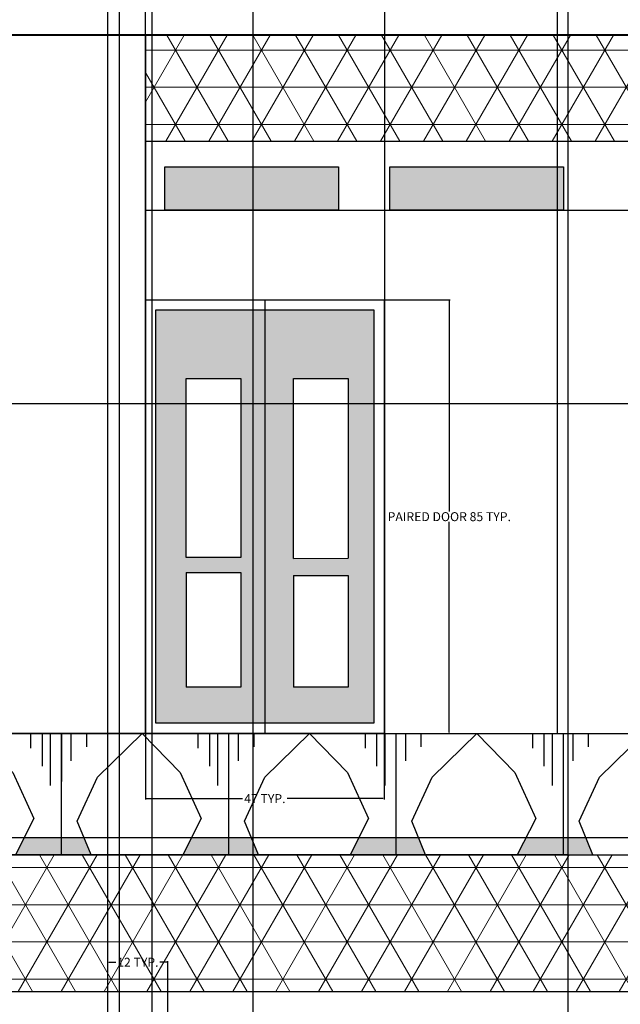
# Model space of a CAD drawing. Units: inches. Extents: x -17 to 741, y 7 to 490.
# Tile 4 of 8: x 254 to 371, y 191 to 383. Entities that reach past the tile are written whole.
import ezdxf

# ---------------------------------------------------------------- set-up
doc = ezdxf.new("R2010")
doc.units = ezdxf.units.IN
doc.header["$MEASUREMENT"] = 0
for name, color, linetype, lineweight in [('A-ANNO-DIMS', 2, 'Continuous', 18), ('A-DOOR', 3, 'Continuous', 25), ('A-ELEV-PATT', 252, 'Continuous', 13), ('A-FLOR-RAIL', 7, 'Continuous', 25), ('A-ROOF-CNPE', 7, 'Continuous', 25), ('A-ROOF-PATT', 8, 'Continuous', 13), ('A-WALL', 7, 'Continuous', 35), ('A-WALL-TRIM', 7, 'Continuous', 25)]:
    doc.layers.add(name, color=color, linetype=linetype, lineweight=lineweight)
doc.styles.get("Standard").update_dxf_attribs({"font": 'arial.ttf'})
doc.dimstyles.get("Standard").update_dxf_attribs({"dimtxt": 1.75, "dimasz": 0.18, "dimexe": 0.18, "dimexo": 0.0625, "dimgap": 0.09, "dimtad": 0, "dimtih": 1, "dimtoh": 1, "dimdec": 4, "dimzin": 0, "dimdsep": 46, "dimlunit": 4, "dimtxsty": 'Standard', "dimcen": 0.09, "dimadec": 0, "dimazin": 0, "dimtfac": 1, "dimtdec": 4, "dimtofl": 0, "dimtmove": 0, "dimatfit": 3, "dimfxl": 1, "dimtolj": 1, "dimtzin": 0, "dimarcsym": 0})

# ---------------------------------------------------------------- blocks, each defined once
blk = doc.blocks.new('BALCONY-POINTED-PANEL')
for p, q in [((0, 23.66), (33.75, 23.66)), ((1.12, 23.66), (1.12, 14.33)), ((2.97, 23.66), (2.97, 18.36)), ((6.01, 23.66), (6.01, 21.09)), ((27.76, 23.66), (27.76, 20.83)), ((29.99, 23.66), (29.99, 17.32)), ((31.57, 23.66), (31.57, 13.51)), ((33.75, 23.66), (33.75, 0))]:
    blk.add_line(p, q)
blk.add_lwpolyline([(6.92, 0), (4.23, 6.57), (8.17, 15.14), (16.88, 23.66), (24.3, 16.07), (28.38, 7.1), (24.8, 0)])
blk = doc.blocks.new('DOOR-PAIR-FRAME')
blk.add_line((23.28, 84.63), (23.28, 0))
for points in [[(0, 84.63), (46.56, 84.63), (46.56, 0), (0, 0)], [(2, 82.63), (44.56, 82.63), (44.56, 2), (2, 2)]]:
    blk.add_lwpolyline(points, close=True)
blk = doc.blocks.new('*D28')
at = {"layer": 'A-ANNO-DIMS', "color": 0, "lineweight": -2, "transparency": 16777216}
for p, q in [((271.44, 179.93), (271.44, 199.23)), ((271.62, 199.05), (273.01, 199.05)), ((282.93, 199.05), (281.54, 199.05)), ((283.11, 179.93), (283.11, 199.23))]:
    blk.add_line(p, q, dxfattribs=at)
at = {"layer": 'A-ANNO-DIMS', "color": 0, "transparency": 16777216}
for points in [[(271.62, 199.08), (271.62, 199.02), (271.44, 199.05)], [(282.93, 199.08), (282.93, 199.02), (283.11, 199.05)]]:
    blk.add_solid(points, dxfattribs=at)
at = {"layer": 'Defpoints', "color": 0, "transparency": 16777216}
for p in [(283.11, 199.05), (271.44, 179.87), (283.11, 179.87)]:
    blk.add_point(p, dxfattribs=at)
at = {"layer": 'A-ANNO-DIMS', "color": 0, "transparency": 16777216, "insert": (277.28, 199.05), "char_height": 1.75, "attachment_point": 5}
blk.add_mtext('\\A1;12 TYP.', dxfattribs=at)
blk = doc.blocks.new('*D29')
at = {"layer": 'A-ANNO-DIMS', "color": 0, "lineweight": -2, "transparency": 16777216}
for p, q in [((325.4, 328.3), (338.21, 328.3)), ((338.03, 328.12), (338.03, 286.98)), ((338.03, 243.85), (338.03, 284.99)), ((325.4, 243.67), (338.21, 243.67))]:
    blk.add_line(p, q, dxfattribs=at)
at = {"layer": 'A-ANNO-DIMS', "color": 0, "transparency": 16777216}
for points in [[(338, 328.12), (338.06, 328.12), (338.03, 328.3)], [(338, 243.85), (338.06, 243.85), (338.03, 243.67)]]:
    blk.add_solid(points, dxfattribs=at)
at = {"layer": 'Defpoints', "color": 0, "transparency": 16777216}
for p in [(325.34, 328.3), (338.03, 328.3), (325.34, 243.67)]:
    blk.add_point(p, dxfattribs=at)
at = {"layer": 'A-ANNO-DIMS', "color": 0, "transparency": 16777216, "insert": (338.03, 285.98), "char_height": 1.75, "attachment_point": 5}
blk.add_mtext('\\A1;PAIRED DOOR 85 TYP.', dxfattribs=at)
blk = doc.blocks.new('*D30')
at = {"layer": 'A-ANNO-DIMS', "color": 0, "lineweight": -2, "transparency": 16777216}
for p, q in [((278.78, 243.61), (278.78, 230.79)), ((325.34, 243.61), (325.34, 230.79)), ((278.96, 230.97), (297.68, 230.97)), ((325.16, 230.97), (306.44, 230.97))]:
    blk.add_line(p, q, dxfattribs=at)
at = {"layer": 'A-ANNO-DIMS', "color": 0, "transparency": 16777216}
for points in [[(278.96, 231), (278.96, 230.94), (278.78, 230.97)], [(325.16, 231), (325.16, 230.94), (325.34, 230.97)]]:
    blk.add_solid(points, dxfattribs=at)
at = {"layer": 'Defpoints', "color": 0, "transparency": 16777216}
for p in [(278.78, 243.67), (325.34, 243.67), (325.34, 230.97)]:
    blk.add_point(p, dxfattribs=at)
at = {"layer": 'A-ANNO-DIMS', "color": 0, "transparency": 16777216, "insert": (302.06, 230.97), "char_height": 1.75, "attachment_point": 5}
blk.add_mtext('\\A1;47 TYP.', dxfattribs=at)
blk = doc.blocks.new('*D37')
at = {"layer": 'A-ANNO-DIMS', "color": 0, "lineweight": -2, "transparency": 16777216}
for p, q in [((20.52, 396.95), (20.52, 14.58)), ((553.43, 51.95), (553.43, 14.58)), ((20.7, 14.76), (283.93, 14.76)), ((553.25, 14.76), (290.02, 14.76))]:
    blk.add_line(p, q, dxfattribs=at)
at = {"layer": 'A-ANNO-DIMS', "color": 0, "transparency": 16777216}
for points in [[(20.7, 14.79), (20.7, 14.73), (20.52, 14.76)], [(553.25, 14.79), (553.25, 14.73), (553.43, 14.76)]]:
    blk.add_solid(points, dxfattribs=at)
at = {"layer": 'Defpoints', "color": 0, "transparency": 16777216}
for p in [(20.52, 397.01), (553.43, 52.01), (553.43, 14.76)]:
    blk.add_point(p, dxfattribs=at)
at = {"layer": 'A-ANNO-DIMS', "color": 0, "transparency": 16777216, "insert": (286.97, 14.76), "char_height": 1.75, "attachment_point": 5}
blk.add_mtext('\\A1;532.9', dxfattribs=at)
blk = doc.blocks.new('*D38')
at = {"layer": 'A-ANNO-DIMS', "color": 0, "lineweight": -2, "transparency": 16777216}
for p, q in [((341.83, 454.57), (723.06, 454.57)), ((722.88, 454.39), (722.88, 254.27)), ((722.88, 52.19), (722.88, 252.31)), ((553.49, 52.01), (723.06, 52.01))]:
    blk.add_line(p, q, dxfattribs=at)
at = {"layer": 'A-ANNO-DIMS', "color": 0, "transparency": 16777216}
for points in [[(722.85, 454.39), (722.91, 454.39), (722.88, 454.57)], [(722.85, 52.19), (722.91, 52.19), (722.88, 52.01)]]:
    blk.add_solid(points, dxfattribs=at)
at = {"layer": 'Defpoints', "color": 0, "transparency": 16777216}
for p in [(341.77, 454.57), (722.88, 454.57), (553.43, 52.01)]:
    blk.add_point(p, dxfattribs=at)
at = {"layer": 'A-ANNO-DIMS', "color": 0, "transparency": 16777216, "insert": (722.88, 253.29), "char_height": 1.75, "attachment_point": 5}
blk.add_mtext('\\A1;402.6', dxfattribs=at)
blk = doc.blocks.new('*D47')
at = {"layer": 'A-ANNO-DIMS', "color": 0, "lineweight": -2, "transparency": 16777216}
for p, q in [((493.03, 379.95), (-13.46, 379.95)), ((-13.28, 379.77), (-13.28, 344.94)), ((-13.28, 308.15), (-13.28, 342.97)), ((553.37, 307.97), (-13.46, 307.97))]:
    blk.add_line(p, q, dxfattribs=at)
at = {"layer": 'A-ANNO-DIMS', "color": 0, "transparency": 16777216}
for points in [[(-13.31, 379.77), (-13.25, 379.77), (-13.28, 379.95)], [(-13.31, 308.15), (-13.25, 308.15), (-13.28, 307.97)]]:
    blk.add_solid(points, dxfattribs=at)
at = {"layer": 'Defpoints', "color": 0, "transparency": 16777216}
for p in [(493.1, 379.95), (-13.28, 307.97), (553.43, 307.97)]:
    blk.add_point(p, dxfattribs=at)
at = {"layer": 'A-ANNO-DIMS', "color": 0, "transparency": 16777216, "insert": (-13.28, 343.96), "char_height": 1.75, "attachment_point": 5}
blk.add_mtext('\\A1;71.98', dxfattribs=at)
blk = doc.blocks.new('*D52')
at = {"layer": 'A-ANNO-DIMS', "color": 0, "lineweight": -2, "transparency": 16777216}
for p, q in [((239.94, 113.25), (239.94, 488.55)), ((240.12, 488.37), (253.76, 488.37)), ((273.51, 488.37), (259.86, 488.37)), ((273.69, 113.25), (273.69, 488.55))]:
    blk.add_line(p, q, dxfattribs=at)
at = {"layer": 'A-ANNO-DIMS', "color": 0, "transparency": 16777216}
for points in [[(240.12, 488.4), (240.12, 488.34), (239.94, 488.37)], [(273.51, 488.4), (273.51, 488.34), (273.69, 488.37)]]:
    blk.add_solid(points, dxfattribs=at)
at = {"layer": 'Defpoints', "color": 0, "transparency": 16777216}
for p in [(273.69, 488.37), (239.94, 113.19), (273.69, 113.19)]:
    blk.add_point(p, dxfattribs=at)
at = {"layer": 'A-ANNO-DIMS', "color": 0, "transparency": 16777216, "insert": (256.81, 488.37), "char_height": 1.75, "attachment_point": 5}
blk.add_mtext('\\A1;33.75', dxfattribs=at)
blk = doc.blocks.new('*D53')
at = {"layer": 'A-ANNO-DIMS', "color": 0, "lineweight": -2, "transparency": 16777216}
for p, q in [((271.44, 167.89), (271.44, 488.55)), ((271.62, 488.37), (361.78, 488.37)), ((457.87, 488.37), (367.7, 488.37)), ((458.05, 167.89), (458.05, 488.55))]:
    blk.add_line(p, q, dxfattribs=at)
at = {"layer": 'A-ANNO-DIMS', "color": 0, "transparency": 16777216}
for points in [[(271.62, 488.4), (271.62, 488.34), (271.44, 488.37)], [(457.87, 488.4), (457.87, 488.34), (458.05, 488.37)]]:
    blk.add_solid(points, dxfattribs=at)
at = {"layer": 'Defpoints', "color": 0, "transparency": 16777216}
for p in [(458.05, 488.37), (271.44, 167.83), (458.05, 167.83)]:
    blk.add_point(p, dxfattribs=at)
at = {"layer": 'A-ANNO-DIMS', "color": 0, "transparency": 16777216, "insert": (364.74, 488.37), "char_height": 1.75, "attachment_point": 5}
blk.add_mtext('\\A1;186.6', dxfattribs=at)
blk = doc.blocks.new('*D56')
at = {"layer": 'A-ANNO-DIMS', "color": 0, "lineweight": -2, "transparency": 16777216}
for p, q in [((225.47, 260.11), (225.47, 488.55)), ((225.65, 488.37), (249.25, 488.37)), ((278.6, 488.37), (255, 488.37)), ((278.78, 243.73), (278.78, 488.55))]:
    blk.add_line(p, q, dxfattribs=at)
at = {"layer": 'A-ANNO-DIMS', "color": 0, "transparency": 16777216}
for points in [[(225.65, 488.4), (225.65, 488.34), (225.47, 488.37)], [(278.6, 488.4), (278.6, 488.34), (278.78, 488.37)]]:
    blk.add_solid(points, dxfattribs=at)
at = {"layer": 'Defpoints', "color": 0, "transparency": 16777216}
for p in [(278.78, 488.37), (225.47, 260.05), (278.78, 243.67)]:
    blk.add_point(p, dxfattribs=at)
at = {"layer": 'A-ANNO-DIMS', "color": 0, "transparency": 16777216, "insert": (252.12, 488.37), "char_height": 1.75, "attachment_point": 5}
blk.add_mtext('\\A1;53.31', dxfattribs=at)
blk = doc.blocks.new('*D57')
at = {"layer": 'A-ANNO-DIMS', "color": 0, "lineweight": -2, "transparency": 16777216}
for p, q in [((325.44, 243.73), (325.44, 488.55)), ((325.62, 488.37), (367.57, 488.37)), ((415.6, 488.37), (373.65, 488.37)), ((415.78, 260.11), (415.78, 488.55))]:
    blk.add_line(p, q, dxfattribs=at)
at = {"layer": 'A-ANNO-DIMS', "color": 0, "transparency": 16777216}
for points in [[(325.62, 488.4), (325.62, 488.34), (325.44, 488.37)], [(415.6, 488.4), (415.6, 488.34), (415.78, 488.37)]]:
    blk.add_solid(points, dxfattribs=at)
at = {"layer": 'Defpoints', "color": 0, "transparency": 16777216}
for p in [(415.78, 488.37), (415.78, 260.05), (325.44, 243.67)]:
    blk.add_point(p, dxfattribs=at)
at = {"layer": 'A-ANNO-DIMS', "color": 0, "transparency": 16777216, "insert": (370.61, 488.37), "char_height": 1.75, "attachment_point": 5}
blk.add_mtext('\\A1;90.34', dxfattribs=at)
blk = doc.blocks.new('*D60')
at = {"layer": 'A-ANNO-DIMS', "color": 0, "lineweight": -2, "transparency": 16777216}
for p, q in [((280.05, 68.56), (280.05, 488.55)), ((280.23, 488.37), (286.96, 488.37)), ((299.61, 488.37), (292.87, 488.37)), ((299.79, 76.07), (299.79, 488.55))]:
    blk.add_line(p, q, dxfattribs=at)
at = {"layer": 'A-ANNO-DIMS', "color": 0, "transparency": 16777216}
for points in [[(280.23, 488.4), (280.23, 488.34), (280.05, 488.37)], [(299.61, 488.4), (299.61, 488.34), (299.79, 488.37)]]:
    blk.add_solid(points, dxfattribs=at)
at = {"layer": 'Defpoints', "color": 0, "transparency": 16777216}
for p in [(299.79, 488.37), (299.79, 76.01), (280.05, 68.49)]:
    blk.add_point(p, dxfattribs=at)
at = {"layer": 'A-ANNO-DIMS', "color": 0, "transparency": 16777216, "insert": (289.92, 488.37), "char_height": 1.75, "attachment_point": 5}
blk.add_mtext('\\A1;19.74', dxfattribs=at)
blk = doc.blocks.new('*D62')
at = {"layer": 'A-ANNO-DIMS', "color": 0, "lineweight": -2, "transparency": 16777216}
for p, q in [((225.41, 260.05), (-13.46, 260.05)), ((-13.28, 259.87), (-13.28, 252.84)), ((-13.28, 243.85), (-13.28, 250.87)), ((278.72, 243.67), (-13.46, 243.67))]:
    blk.add_line(p, q, dxfattribs=at)
at = {"layer": 'A-ANNO-DIMS', "color": 0, "transparency": 16777216}
for points in [[(-13.31, 259.87), (-13.25, 259.87), (-13.28, 260.05)], [(-13.31, 243.85), (-13.25, 243.85), (-13.28, 243.67)]]:
    blk.add_solid(points, dxfattribs=at)
at = {"layer": 'Defpoints', "color": 0, "transparency": 16777216}
for p in [(225.47, 260.05), (-13.28, 243.67), (278.78, 243.67)]:
    blk.add_point(p, dxfattribs=at)
at = {"layer": 'A-ANNO-DIMS', "color": 0, "transparency": 16777216, "insert": (-13.28, 251.86), "char_height": 1.75, "attachment_point": 5}
blk.add_mtext('\\A1;16.38', dxfattribs=at)
blk = doc.blocks.new('*D67')
at = {"layer": 'A-ANNO-DIMS', "color": 0, "lineweight": -2, "transparency": 16777216}
for p, q in [((359.14, 243.73), (359.14, 488.55)), ((359.32, 488.37), (372.41, 488.37)), ((391.59, 488.37), (378.49, 488.37)), ((391.77, 243.73), (391.77, 488.55))]:
    blk.add_line(p, q, dxfattribs=at)
at = {"layer": 'A-ANNO-DIMS', "color": 0, "transparency": 16777216}
for points in [[(359.32, 488.4), (359.32, 488.34), (359.14, 488.37)], [(391.59, 488.4), (391.59, 488.34), (391.77, 488.37)]]:
    blk.add_solid(points, dxfattribs=at)
at = {"layer": 'Defpoints', "color": 0, "transparency": 16777216}
for p in [(391.77, 488.37), (359.14, 243.67), (391.77, 243.67)]:
    blk.add_point(p, dxfattribs=at)
at = {"layer": 'A-ANNO-DIMS', "color": 0, "transparency": 16777216, "insert": (375.45, 488.37), "char_height": 1.75, "attachment_point": 5}
blk.add_mtext('\\A1;32.63', dxfattribs=at)
blk = doc.blocks.new('*D68')
at = {"layer": 'A-ANNO-DIMS', "color": 0, "lineweight": -2, "transparency": 16777216}
for p, q in [((280.05, 61.98), (280.05, 488.55)), ((280.23, 488.37), (317.59, 488.37)), ((361.04, 488.37), (323.68, 488.37)), ((361.22, 61.98), (361.22, 488.55))]:
    blk.add_line(p, q, dxfattribs=at)
at = {"layer": 'A-ANNO-DIMS', "color": 0, "transparency": 16777216}
for points in [[(280.23, 488.4), (280.23, 488.34), (280.05, 488.37)], [(361.04, 488.4), (361.04, 488.34), (361.22, 488.37)]]:
    blk.add_solid(points, dxfattribs=at)
at = {"layer": 'Defpoints', "color": 0, "transparency": 16777216}
for p in [(361.22, 488.37), (280.05, 61.91), (361.22, 61.91)]:
    blk.add_point(p, dxfattribs=at)
at = {"layer": 'A-ANNO-DIMS', "color": 0, "transparency": 16777216, "insert": (320.64, 488.37), "char_height": 1.75, "attachment_point": 5}
blk.add_mtext('\\A1;81.18', dxfattribs=at)

msp = doc.modelspace()

# ---------------------------------------------------------------- hatches: boundary and pattern name
at = {"layer": 'A-ELEV-PATT'}
h = msp.add_hatch(dxfattribs=at)
h.set_pattern_fill('STARS', color=256, scale=19)
h.paths.add_polyline_path([(204.6793, 330.2905), (174.1219, 330.2905), (174.1219, 324.7204), (204.6793, 324.7204)])
h.paths.add_polyline_path([(238.7618, 330.6251), (208.2044, 330.6251), (208.2044, 325.055), (238.7618, 325.055)])
h.paths.add_polyline_path([(316.4391, 354.2167), (282.5434, 354.2167), (282.5434, 345.7496), (316.4391, 345.7496)])
h.paths.add_polyline_path([(360.3395, 354.2167), (326.4438, 354.2167), (326.4438, 345.7496), (360.3395, 345.7496)])
h.paths.add_polyline_path([(407.6938, 354.2167), (373.7981, 354.2167), (373.7981, 345.7496), (407.6938, 345.7496)])
h.paths.add_polyline_path([(290.7055, 188.3373), (256.8098, 188.3373), (256.8098, 179.8702), (290.7055, 179.8702)])
h.paths.add_polyline_path([(332.372, 188.3373), (298.4763, 188.3373), (298.4763, 179.8702), (332.372, 179.8702)])
h.paths.add_polyline_path([(375.4339, 188.3373), (341.5382, 188.3373), (341.5382, 179.8702), (375.4339, 179.8702)])
h.paths.add_polyline_path([(419.3343, 188.3373), (385.4386, 188.3373), (385.4386, 179.8702), (419.3343, 179.8702)])
h.paths.add_polyline_path([(466.6886, 188.3373), (432.7929, 188.3373), (432.7929, 179.8702), (466.6886, 179.8702)])
h = msp.add_hatch(color=256, dxfattribs=at)
h.dxf.hatch_style = 1
h.paths.add_polyline_path([(323.3398, 326.2997), (302.06, 326.2997), (302.06, 245.669), (323.3398, 245.669)])
h.paths.add_polyline_path([(318.294, 312.92), (318.294, 277.8507), (307.6578, 277.839), (307.6578, 312.92)], flags=16)
h.paths.add_polyline_path([(318.294, 274.5229), (318.294, 252.6962), (307.6578, 252.6962), (307.6578, 274.5229)], flags=16)
h.paths.add_polyline_path([(302.06, 326.2997), (280.7803, 326.2997), (280.7803, 245.669), (302.06, 245.669)])
h.paths.add_polyline_path([(297.3761, 312.92), (297.3761, 278.0199), (286.7398, 278.0199), (286.7398, 312.92)], flags=16)
h.paths.add_polyline_path([(297.3761, 275.0626), (297.3761, 252.6962), (286.7398, 252.6962), (286.7398, 275.0626)], flags=16)
h = msp.add_hatch(color=256, dxfattribs=at)
h.dxf.hatch_style = 1
h.paths.add_polyline_path([(103.6141, 223.3801), (98.075, 223.3801), (98.075, 220.0082), (104.992, 220.0082)])
h.paths.add_polyline_path([(131.8275, 223.3801), (124.5765, 223.3801), (122.878, 220.0082), (131.8275, 220.0082)])
h.paths.add_polyline_path([(136.2468, 223.3801), (131.8275, 223.3801), (131.8275, 220.0082), (137.6247, 220.0082)])
h.paths.add_polyline_path([(164.4602, 223.3801), (157.2092, 223.3801), (155.5107, 220.0082), (164.4602, 220.0082)])
h.paths.add_polyline_path([(168.8795, 223.3801), (164.4602, 223.3801), (164.4602, 220.0082), (170.2574, 220.0082)])
h.paths.add_polyline_path([(197.0929, 223.3801), (189.8419, 223.3801), (188.1434, 220.0082), (197.0929, 220.0082)])
h.paths.add_polyline_path([(201.5121, 223.3801), (197.0929, 223.3801), (197.0929, 220.0082), (202.8901, 220.0082)])
h.paths.add_polyline_path([(229.7256, 223.3801), (222.4746, 223.3801), (220.776, 220.0082), (229.7256, 220.0082)])
h.paths.add_polyline_path([(234.1448, 223.3801), (229.7256, 223.3801), (229.7256, 220.0082), (235.5227, 220.0082)])
h.paths.add_polyline_path([(262.3583, 223.3801), (255.1072, 223.3801), (253.4087, 220.0082), (262.3583, 220.0082)])
h.paths.add_polyline_path([(266.7775, 223.3801), (262.3583, 223.3801), (262.3583, 220.0082), (268.1554, 220.0082)])
h.paths.add_polyline_path([(294.9909, 223.3801), (287.7399, 223.3801), (286.0414, 220.0082), (294.9909, 220.0082)])
h.paths.add_polyline_path([(299.4102, 223.3801), (294.9909, 223.3801), (294.9909, 220.0082), (300.7881, 220.0082)])
h.paths.add_polyline_path([(327.6236, 223.3801), (320.3726, 223.3801), (318.6741, 220.0082), (327.6236, 220.0082)])
h.paths.add_polyline_path([(332.0429, 223.3801), (327.6236, 223.3801), (327.6236, 220.0082), (333.4208, 220.0082)])
h.paths.add_polyline_path([(360.2563, 223.3801), (353.0053, 223.3801), (351.3068, 220.0082), (360.2563, 220.0082)])
h.paths.add_polyline_path([(364.6755, 223.3801), (360.2563, 223.3801), (360.2563, 220.0082), (361.2234, 220.0082), (366.0535, 220.0082)])
h.paths.add_polyline_path([(392.889, 223.3801), (385.638, 223.3801), (383.9394, 220.0082), (392.889, 220.0082)])
h.paths.add_polyline_path([(397.3082, 223.3801), (392.889, 223.3801), (392.889, 220.0082), (398.6861, 220.0082)])
h.paths.add_polyline_path([(425.5216, 223.3801), (418.2706, 223.3801), (416.5721, 220.0082), (425.5216, 220.0082)])
h.paths.add_polyline_path([(429.9409, 223.3801), (425.5216, 223.3801), (425.5216, 220.0082), (431.3188, 220.0082)])
h.paths.add_polyline_path([(458.1543, 223.3801), (450.9033, 223.3801), (449.2048, 220.0082), (458.1543, 220.0082)])
at = {"layer": 'A-ROOF-PATT'}
h = msp.add_hatch(dxfattribs=at)
h.set_pattern_fill('NET3', color=256, scale=58)
h.paths.add_polyline_path([(478.3168, 220.0082), (470.3932, 220.0082), (361.2234, 220.0082), (239.9367, 220.0082), (229.7523, 193.3539), (470.754, 193.3539), (488.0578, 193.3539)])
h.paths.add_polyline_path([(421.4932, 379.9466), (278.7803, 379.9466), (278.7803, 359.2334), (411.7592, 359.2334), (429.063, 359.2334)])

# ---------------------------------------------------------------- linework, layer by layer
at = {"layer": 'A-DOOR'}
for p, q in [((286.7398, 312.92), (297.3761, 312.92)), ((286.7398, 278.0199), (286.7398, 312.92)), ((297.3761, 312.92), (297.3761, 278.0199)), ((307.6578, 312.92), (318.294, 312.92)), ((307.6578, 277.839), (307.6578, 312.92)), ((318.294, 312.92), (318.294, 277.8507)), ((297.3761, 278.0199), (286.7398, 278.0199)), ((307.6578, 277.839), (318.294, 277.8507)), ((286.7398, 275.0626), (297.3761, 275.0626)), ((286.7398, 275.0626), (286.7398, 252.6962)), ((297.3761, 275.0626), (297.3761, 252.6962)), ((307.6578, 274.5229), (318.294, 274.5229)), ((307.6578, 274.5229), (307.6578, 252.6962)), ((318.294, 274.5229), (318.294, 252.6962)), ((297.3761, 252.6962), (286.7398, 252.6962)), ((318.294, 252.6962), (307.6578, 252.6962))]:
    msp.add_line(p, q, dxfattribs=at)
at = {"layer": 'A-FLOR-RAIL'}
msp.add_line((98.075, 223.3801), (478.3168, 223.3801), dxfattribs=at)
at = {"layer": 'A-ROOF-CNPE'}
msp.add_line((278.7803, 345.7496), (407.6938, 345.7496), dxfattribs=at)
msp.add_line((278.7803, 345.7496), (407.6938, 345.7496), dxfattribs=at)
for points in [[(278.7803, 359.2334), (411.7592, 359.2334)], [(278.7803, 359.2334), (411.7592, 359.2334)], [(239.9367, 220.0082), (229.7523, 193.3539), (470.754, 193.3539)], [(361.2234, 220.0082), (470.3932, 220.0082)]]:
    msp.add_lwpolyline(points, dxfattribs=at)
for points in [[(282.5434, 354.2167), (316.4391, 354.2167), (316.4391, 345.7496), (282.5434, 345.7496)], [(282.5434, 354.2167), (316.4391, 354.2167), (316.4391, 345.7496), (282.5434, 345.7496)], [(326.4438, 354.2167), (360.3395, 354.2167), (360.3395, 345.7496), (326.4438, 345.7496)], [(326.4438, 354.2167), (360.3395, 354.2167), (360.3395, 345.7496), (326.4438, 345.7496)]]:
    msp.add_lwpolyline(points, close=True, dxfattribs=at)
at = {"layer": 'A-WALL'}
for p, q in [((278.7803, 379.9466), (278.7803, 243.669)), ((98.075, 220.0082), (361.2234, 220.0082))]:
    msp.add_line(p, q, dxfattribs=at)
at = {"layer": 'A-WALL-TRIM'}
msp.add_lwpolyline([(53.4591, 295.9), (53.4591, 295.9), (72.6093, 295.9), (97.1425, 365.3552), (97.1425, 379.9466), (515.96, 379.9466)], dxfattribs=at)

# ---------------------------------------------------------------- block references
at = {"layer": 'A-DOOR'}
msp.add_blockref('DOOR-PAIR-FRAME', (278.7806, 243.6688), dxfattribs=at)
at = {"layer": 'A-FLOR-RAIL'}
for p in [(228.6057, 220.008), (261.2384, 220.008), (293.8711, 220.008), (326.5037, 220.008), (359.1364, 220.008)]:
    msp.add_blockref('BALCONY-POINTED-PANEL', p, dxfattribs=at)

# ---------------------------------------------------------------- dimensions: what is measured, and where the dimension line sits
at = {"layer": 'A-ANNO-DIMS'}
for base, p1, p2, override, picture, middle in [((278.7803, 488.3717), (225.4694, 260.0479), (278.7803, 243.669), {"dimdec": 2, "dimlfac": 1, "dimrnd": 0, "dimzin": 0, "dimdsep": 46, "dimlunit": 2}, '*D56', (252.1249, 488.3717)), ((273.6893, 488.3717), (239.9367, 113.1863), (273.6893, 113.1863), {"dimdec": 2, "dimlfac": 1, "dimrnd": 0, "dimzin": 0, "dimdsep": 46, "dimlunit": 2}, '*D52', (256.813, 488.3717)), ((458.0494, 488.3717), (271.4367, 167.8255), (458.0494, 167.8255), {"dimdec": 1, "dimlfac": 1, "dimrnd": 0, "dimzin": 0, "dimdsep": 46, "dimlunit": 2}, '*D53', (364.743, 488.3717)), ((299.7867, 488.3717), (280.0481, 68.493), (299.7867, 76.0082), {"dimdec": 2, "dimlfac": 1, "dimrnd": 0, "dimzin": 0, "dimdsep": 46, "dimlunit": 2}, '*D60', (289.9174, 488.3717)), ((361.2234, 488.3717), (280.0481, 61.9147), (361.2234, 61.9147), {"dimdec": 2, "dimlfac": 1, "dimrnd": 0, "dimzin": 0, "dimdsep": 46, "dimlunit": 2}, '*D68', (320.6357, 488.3717)), ((415.7774, 488.3717), (325.441, 243.669), (415.7774, 260.0479), {"dimdec": 2, "dimlfac": 1, "dimrnd": 0, "dimzin": 0, "dimdsep": 46, "dimlunit": 2}, '*D57', (370.6092, 488.3717)), ((391.7691, 488.3717), (359.1364, 243.669), (391.7691, 243.669), {"dimdec": 2, "dimlfac": 1, "dimrnd": 0, "dimzin": 0, "dimdsep": 46, "dimlunit": 2}, '*D67', (375.4527, 488.3717)), ((553.4286, 14.7597), (20.5169, 397.0087), (553.4286, 52.0082), {"dimdec": 1, "dimlfac": 1, "dimrnd": 0, "dimzin": 0, "dimdsep": 46, "dimlunit": 2}, '*D37', (286.9727, 14.7597))]:
    dim = msp.add_linear_dim(base=base, p1=p1, p2=p2, dimstyle='Standard', override=override, dxfattribs=at)
    dim.commit()
    dim.dimension.update_dxf_attribs({"geometry": picture, "text_midpoint": middle})
for base, p1, p2, override, picture, middle in [((722.8826, 454.5717), (553.4286, 52.0082), (341.7687, 454.5717), {"dimdec": 1, "dimlfac": 1, "dimrnd": 0, "dimzin": 0, "dimdsep": 46, "dimlunit": 2}, '*D38', (722.8826, 253.2899)), ((-13.2831, 307.9703), (493.0961, 379.9466), (553.4286, 307.9703), {"dimdec": 2, "dimlfac": 1, "dimrnd": 0, "dimzin": 0, "dimdsep": 46, "dimlunit": 2}, '*D47', (-13.2831, 343.9584)), ((-13.2831, 243.669), (225.4694, 260.0479), (278.7803, 243.669), {"dimdec": 2, "dimlfac": 1, "dimrnd": 0, "dimzin": 0, "dimdsep": 46, "dimlunit": 2}, '*D62', (-13.2831, 251.8584))]:
    dim = msp.add_linear_dim(base=base, p1=p1, p2=p2, angle=90, dimstyle='Standard', override=override, dxfattribs=at)
    dim.commit()
    dim.dimension.update_dxf_attribs({"geometry": picture, "text_midpoint": middle})
dim = msp.add_linear_dim(base=(338.0344, 328.2997), p1=(325.3398, 243.669), p2=(325.3398, 328.2997), angle=90, text='PAIRED DOOR <> TYP.', dimstyle='Standard', override={"dimdec": 0, "dimlfac": 1, "dimrnd": 0, "dimzin": 0, "dimdsep": 46, "dimlunit": 2}, dxfattribs=at)
dim.commit()
dim.dimension.update_dxf_attribs({"geometry": '*D29', "text_midpoint": (338.0344, 285.9843)})
for base, p1, p2, picture, middle in [((325.3398, 230.9743), (278.7803, 243.669), (325.3398, 243.669), '*D30', (302.06, 230.9743)), ((283.1138, 199.0495), (271.4367, 179.8702), (283.1138, 179.8702), '*D28', (277.2752, 199.0495))]:
    dim = msp.add_linear_dim(base=base, p1=p1, p2=p2, text='<> TYP.', dimstyle='Standard', override={"dimdec": 0, "dimlfac": 1, "dimrnd": 0, "dimzin": 0, "dimdsep": 46, "dimlunit": 2}, dxfattribs=at)
    dim.commit()
    dim.dimension.update_dxf_attribs({"geometry": picture, "text_midpoint": middle})

doc.saveas('drawing.dxf')
